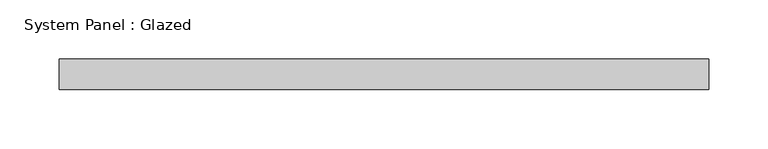
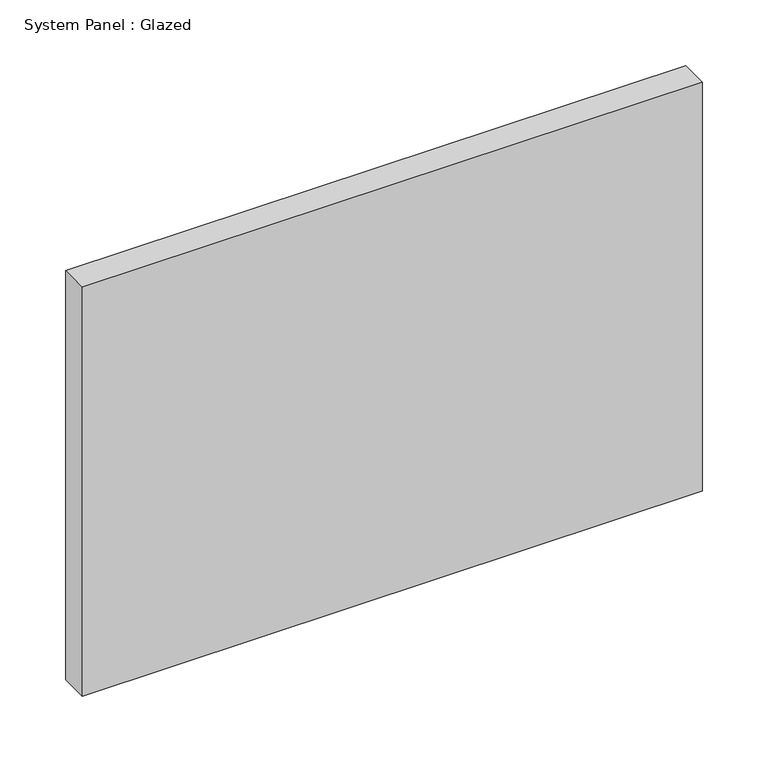
"""IFC4 building model written with IfcOpenShell, lengths in millimetres: plate geometry, System Panel : Glazed."""

from ifc_helpers import new_model, si_unit, origin, origin_with_axes, place, context, project, spatial, polyline, outline, extrude, source, transform, mapped, element, save


def system_panel_glazed_86de8a05(model_context):
    return source(origin(), model_context, "Body", "SweptSolid", [
        extrude(outline(polyline([(273.05, 19.05), (-273.05, 19.05), (-273.05, 44.45), (273.05, 44.45), (273.05, 19.05)])), origin_with_axes(), (0.0, 0.0, 1.0), 381.0),
    ])


if __name__ == "__main__":
    model = new_model("IFC4")
    model_context = context("Model", 3, world=origin())
    ifc_project = project(units=[si_unit("LENGTHUNIT", "METRE", prefix="MILLI")], contexts=[model_context])
    site = spatial("IfcSite", under=ifc_project)
    building = spatial("IfcBuilding", under=site)
    placement = place(None, origin())
    system_panel_glazed_shape = system_panel_glazed_86de8a05(model_context)
    element("IfcPlate", 1, ObjectType="System Panel : Glazed", at=placement, inside=building, context=model_context, shape_type="MappedRepresentation", body=[
        mapped(system_panel_glazed_shape, transform((0.0, 0.0, 0.0), x_axis=(1.0, 0.0, 0.0), y_axis=(0.0, 1.0, 0.0), z_axis=(0.0, 0.0, 1.0))),
    ])
    save(model, "model.ifc")

# Revit data of these elements
# Type "System Panel : Glazed"
#   Construction Type Id = "GSP4R"
#   Analytic Construction = "1/8 in Pilkington single glazing"
#   Visual Light Transmittance = 0.9
#   Solar Heat Gain Coefficient = 0.86
#   Heat Transfer Coefficient (U) = 1.18115 BTU/(h·ft²·°F)
#   Define Thermal Properties by = 1
# Element 1 (IfcPlate, "System Panel : Glazed")
#   Materials on its faces: "Glass"
# Materials
#   "Glass": class "Glass", colour RGB 0 128 192, transparency 0.75, Description = "Soda Lime Glass", Cost = 0
